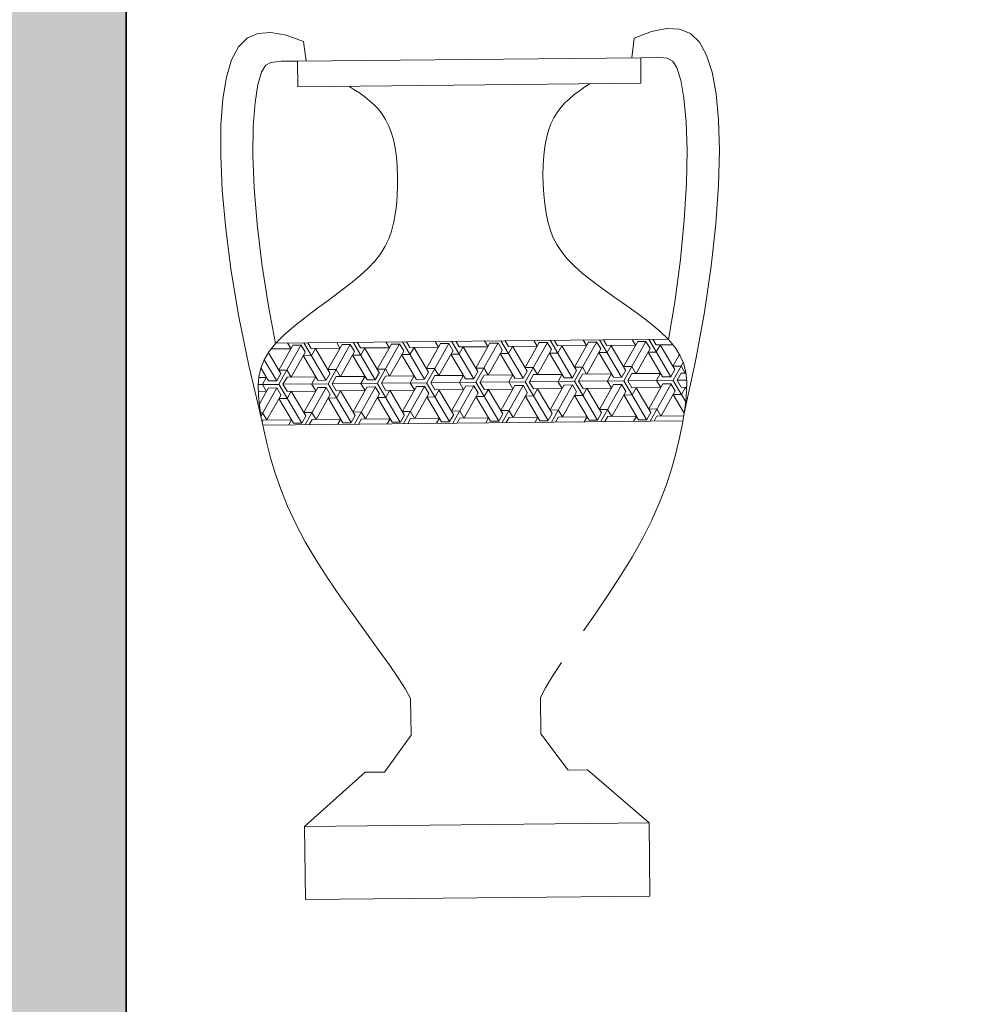
# Model space of a CAD drawing. Units: inches. Extents: x 638 to 1303, y 1 to 699.
# Tile 15 of 21: x 924.49 to 944.42, y 576.64 to 597.47. Entities that reach past the tile are written whole.
import ezdxf

# ---------------------------------------------------------------- set-up
doc = ezdxf.new("R2010")
doc.units = ezdxf.units.IN
doc.header["$MEASUREMENT"] = 0
doc.layers.add('A-FURN-ACCS', color=8, linetype='Continuous', lineweight=13)
doc.layers.add('A-WALL', color=7, linetype='Continuous', lineweight=35)
doc.layers.add('A-WALL-PATT', color=143, linetype='Continuous', lineweight=13, true_color=0x7aafdf)

msp = doc.modelspace()

# ---------------------------------------------------------------- hatches: boundary and pattern name
at = {"layer": 'A-WALL-PATT'}
h = msp.add_hatch(color=256, dxfattribs=at)
h.dxf.hatch_style = 1
h.paths.add_polyline_path([(973.34524, 629.81895), (793.35541, 629.81895), (793.35541, 620.81895), (850.23798, 620.81895), (922.23798, 620.81895), (922.23798, 524.81895), (908.94335, 524.81895), (908.94335, 520.31895), (926.73798, 520.31895), (926.73798, 544.31895), (979.3571, 544.31895), (979.3571, 548.81895), (926.73798, 548.81895), (926.73798, 620.81895), (973.34524, 620.81895)])
h.paths.add_polyline_path([(758.35541, 629.81895), (697.23798, 629.81895), (697.23798, 586.77451), (706.23798, 586.77451), (706.23798, 620.81895), (758.35541, 620.81895)])
h.paths.add_polyline_path([(1075.85281, 629.81895), (1003.34524, 629.81895), (1003.34524, 620.81895), (1046.73798, 620.81895), (1046.73798, 560.81895), (1046.73798, 548.81895), (1026.3571, 548.81895), (1026.3571, 544.31895), (1046.73798, 544.31895), (1046.73798, 486.87457), (1051.23798, 486.87457), (1051.23798, 556.31895), (1162.89753, 556.31895), (1162.89753, 560.81895), (1051.23798, 560.81895), (1051.23798, 620.81895), (1075.85281, 620.81895)])
h.paths.add_polyline_path([(1228.23798, 629.81895), (1105.85281, 629.81895), (1105.85281, 620.81895), (1219.23798, 620.81895), (1219.23798, 560.81895), (1197.89753, 560.81895), (1197.89753, 556.31895), (1219.23798, 556.31895), (1219.23798, 498.80084), (1228.23798, 498.80084)])
h.paths.add_polyline_path([(1051.23798, 439.87457), (1046.73798, 439.87457), (1046.73798, 407.81895), (1219.23798, 407.81895), (1219.23798, 381.66175), (1228.23798, 381.66175), (1228.23798, 451.80084), (1219.23798, 451.80084), (1219.23798, 412.31895), (1051.23798, 412.31895)])
h.paths.add_polyline_path([(1228.23798, 346.66175), (1219.23798, 346.66175), (1219.23798, 335.81895), (1046.73798, 335.81895), (1046.73798, 273.56895), (1051.23798, 273.56895), (1051.23798, 331.31895), (1219.23798, 331.31895), (1219.23798, 308.99654), (1228.23798, 308.99654)])
h.paths.add_polyline_path([(1228.23798, 261.99654), (1219.23798, 261.99654), (1219.23798, 211.31895), (1051.23798, 211.31895), (1051.23798, 226.56895), (1046.73798, 226.56895), (1046.73798, 211.31895), (983.84714, 211.31895), (983.84714, 206.81895), (1219.23798, 206.81895), (1219.23798, 166.83987), (1228.23798, 166.83987)])
h.paths.add_polyline_path([(1228.23798, 119.83987), (1219.23798, 119.83987), (1219.23798, 50.81895), (1197.89277, 50.81895), (1197.89277, 41.81895), (1228.23798, 41.81895)])
h.paths.add_polyline_path([(1162.89277, 50.81895), (1069.02949, 50.81895), (1069.02949, 41.81895), (1162.89277, 41.81895)])
h.paths.add_polyline_path([(1010.02949, 50.81895), (941.89631, 50.81895), (917.77455, 50.81895), (917.77455, 41.81895), (941.89631, 41.81895), (1010.02949, 41.81895)])
h.paths.add_polyline_path([(882.77455, 50.81895), (854.73798, 50.81895), (854.73798, 145.50379), (850.23798, 145.50379), (850.23798, 50.81895), (793.49755, 50.81895), (793.49755, 41.81895), (882.77455, 41.81895)])
h.paths.add_polyline_path([(746.49755, 50.81895), (706.23798, 50.81895), (706.23798, 96.57416), (697.23798, 96.57416), (697.23798, 41.81895), (746.49755, 41.81895)])
h.paths.add_polyline_path([(706.23798, 206.81895), (714.01165, 206.81895), (714.01165, 211.31895), (706.23798, 211.31895), (706.23798, 251.21966), (697.23798, 251.21966), (697.23798, 143.57416), (706.23798, 143.57416)])
h.paths.add_polyline_path([(923.84714, 211.31895), (854.73798, 211.31895), (854.73798, 397.8313), (850.23798, 397.8313), (850.23798, 388.31895), (747.9539, 388.31895), (747.9539, 383.81895), (850.23798, 383.81895), (850.23798, 311.81895), (706.23798, 311.81895), (706.23798, 342.78787), (697.23798, 342.78787), (697.23798, 281.21966), (706.23798, 281.21966), (706.23798, 307.31895), (850.23798, 307.31895), (850.23798, 211.31895), (749.01165, 211.31895), (749.01165, 206.81895), (850.23798, 206.81895), (850.23798, 192.50379), (854.73798, 192.50379), (854.73798, 206.81895), (923.84714, 206.81895)])
h.paths.add_polyline_path([(706.23798, 434.70471), (697.23798, 434.70471), (697.23798, 372.78787), (706.23798, 372.78787), (706.23798, 383.81895), (712.9539, 383.81895), (712.9539, 388.31895), (706.23798, 388.31895)])
h.paths.add_polyline_path([(706.23798, 520.31895), (850.23798, 520.31895), (850.23798, 444.8313), (854.73798, 444.8313), (854.73798, 520.31895), (861.94335, 520.31895), (861.94335, 524.81895), (706.23798, 524.81895), (706.23798, 551.77451), (697.23798, 551.77451), (697.23798, 481.70471), (706.23798, 481.70471)])

# ---------------------------------------------------------------- linework, layer by layer
at = {"layer": 'A-FURN-ACCS'}
for p, q in [((929.29851, 597.0812, 30.93634), (929.52655, 597.18264, 30.93634)), ((929.52655, 597.18264, 30.93634), (929.79966, 597.20234, 30.93634)), ((929.79966, 597.20234, 30.93634), (930.12044, 597.14336, 30.93634)), ((937.85335, 597.22234, 30.93634), (937.48516, 597.08018, 30.93634)), ((938.17285, 597.28786, 30.93634), (937.85335, 597.22234, 30.93634)), ((938.44632, 597.27375, 30.93634), (938.17285, 597.28786, 30.93634)), ((938.67638, 597.17698, 30.93634), (938.44632, 597.27375, 30.93634)), ((938.86569, 596.99458, 30.93634), (938.67638, 597.17698, 30.93634)), ((929.11296, 596.89496, 30.93634), (929.29851, 597.0812, 30.93634)), ((930.12044, 597.14336, 30.93634), (930.49145, 597.00875, 30.93634)), ((930.49145, 597.00875, 30.93634), (930.54731, 596.59361, 30.93634)), ((937.48516, 597.08018, 30.93634), (937.43779, 596.66399, 30.93634)), ((939.01689, 596.72351, 30.93634), (938.86569, 596.99458, 30.93634)), ((928.96733, 596.62087, 30.93634), (929.11296, 596.89496, 30.93634)), ((928.85903, 596.25587, 30.93634), (928.96733, 596.62087, 30.93634)), ((929.69512, 596.50919, 30.93634), (929.80088, 596.56912, 30.93634)), ((929.80088, 596.56912, 30.93634), (930.01698, 596.59481, 30.93634)), ((930.01698, 596.59481, 30.93634), (930.36281, 596.59173, 30.93634)), ((930.36281, 596.59173, 30.93634), (933.99255, 596.6288, 30.93634)), ((930.36831, 596.05264, 30.93634), (930.36281, 596.59173, 30.93634)), ((937.6223, 596.66587, 30.93634), (933.99255, 596.6288, 30.93634)), ((937.968, 596.67602, 30.93634), (937.6223, 596.66587, 30.93634)), ((937.62781, 596.12679, 30.93634), (937.6223, 596.66587, 30.93634)), ((938.18458, 596.65474, 30.93634), (937.968, 596.67602, 30.93634)), ((938.29153, 596.59699, 30.93634), (938.18458, 596.65474, 30.93634)), ((938.29373, 596.59607, 30.93634), (938.29153, 596.59699, 30.93634)), ((938.31801, 596.57267, 30.93634), (938.29373, 596.59607, 30.93634)), ((938.38627, 596.45029, 30.93634), (938.31801, 596.57267, 30.93634)), ((939.13263, 596.3608, 30.93634), (939.01689, 596.72351, 30.93634)), ((929.52722, 596.10387, 30.93634), (929.6034, 596.36059, 30.93634)), ((929.6034, 596.36059, 30.93634), (929.66915, 596.48434, 30.93634)), ((929.66915, 596.48434, 30.93634), (929.69295, 596.50823, 30.93634)), ((929.69295, 596.50823, 30.93634), (929.69512, 596.50919, 30.93634)), ((938.46767, 596.19518, 30.93634), (938.38627, 596.45029, 30.93634)), ((939.21554, 595.90342, 30.93634), (939.13263, 596.3608, 30.93634)), ((928.78547, 595.79689, 30.93634), (928.85903, 596.25587, 30.93634)), ((938.53745, 595.81025, 30.93634), (938.46767, 596.19518, 30.93634)), ((929.46532, 595.71759, 30.93634), (929.52722, 596.10387, 30.93634)), ((937.62781, 596.12679, 30.93634), (930.36831, 596.05264, 30.93634)), ((931.55847, 595.99769, 30.93634), (931.44982, 596.06369, 30.93634)), ((931.67465, 595.92083, 30.93634), (931.55847, 595.99769, 30.93634)), ((936.21523, 595.88586, 30.93634), (936.32443, 595.96832, 30.93634)), ((936.32443, 595.96832, 30.93634), (936.43902, 596.04754, 30.93634)), ((936.43902, 596.04754, 30.93634), (936.5463, 596.11574, 30.93634)), ((928.74499, 595.24222, 30.93634), (928.78547, 595.79689, 30.93634)), ((929.42832, 595.21387, 30.93634), (929.46532, 595.71759, 30.93634)), ((931.78552, 595.84061, 30.93634), (931.67465, 595.92083, 30.93634)), ((931.88949, 595.75738, 30.93634), (931.78552, 595.84061, 30.93634)), ((931.98601, 595.66959, 30.93634), (931.88949, 595.75738, 30.93634)), ((936.01827, 595.71078, 30.93634), (936.11298, 595.80052, 30.93634)), ((936.11298, 595.80052, 30.93634), (936.21523, 595.88586, 30.93634)), ((938.58474, 595.30739, 30.93634), (938.53745, 595.81025, 30.93634)), ((939.26735, 595.34969, 30.93634), (939.21554, 595.90342, 30.93634)), ((932.07478, 595.57522, 30.93634), (931.98601, 595.66959, 30.93634)), ((932.1555, 595.47224, 30.93634), (932.07478, 595.57522, 30.93634)), ((935.78282, 595.39495, 30.93634), (935.85285, 595.51, 30.93634)), ((935.85285, 595.51, 30.93634), (935.93144, 595.61461, 30.93634)), ((935.93144, 595.61461, 30.93634), (936.01827, 595.71078, 30.93634)), ((932.22786, 595.35864, 30.93634), (932.1555, 595.47224, 30.93634)), ((932.29156, 595.23239, 30.93634), (932.22786, 595.35864, 30.93634)), ((935.72171, 595.26743, 30.93634), (935.78282, 595.39495, 30.93634)), ((938.60375, 594.70267, 30.93634), (938.58474, 595.30739, 30.93634)), ((939.28607, 594.70319, 30.93634), (939.26735, 595.34969, 30.93634)), ((928.73948, 594.59548, 30.93634), (928.74499, 595.24222, 30.93634)), ((929.42167, 594.60889, 30.93634), (929.42832, 595.21387, 30.93634)), ((932.3463, 595.09149, 30.93634), (932.29156, 595.23239, 30.93634)), ((932.39177, 594.9339, 30.93634), (932.3463, 595.09149, 30.93634)), ((935.62762, 594.96695, 30.93634), (935.66987, 595.12543, 30.93634)), ((935.66987, 595.12543, 30.93634), (935.72171, 595.26743, 30.93634)), ((932.42776, 594.75862, 30.93634), (932.39177, 594.9339, 30.93634)), ((935.59522, 594.79097, 30.93634), (935.62762, 594.96695, 30.93634)), ((932.4544, 594.56868, 30.93634), (932.42776, 594.75862, 30.93634)), ((935.57246, 594.60053, 30.93634), (935.59522, 594.79097, 30.93634)), ((938.5911, 594.00917, 30.93634), (938.60375, 594.70267, 30.93634)), ((939.2688, 593.96883, 30.93634), (939.28607, 594.70319, 30.93634)), ((928.77174, 593.86162, 30.93634), (928.73948, 594.59548, 30.93634)), ((929.44847, 593.91579, 30.93634), (929.42167, 594.60889, 30.93634)), ((932.47192, 594.36811, 30.93634), (932.4544, 594.56868, 30.93634)), ((935.55904, 594.39964, 30.93634), (935.57246, 594.60053, 30.93634)), ((932.48054, 594.16097, 30.93634), (932.47192, 594.36811, 30.93634)), ((935.55466, 594.19236, 30.93634), (935.55904, 594.39964, 30.93634)), ((932.48047, 593.95127, 30.93634), (932.48054, 594.16097, 30.93634)), ((935.55902, 593.98272, 30.93634), (935.55466, 594.19236, 30.93634)), ((928.84459, 593.0456, 30.93634), (928.77174, 593.86162, 30.93634)), ((929.51085, 593.14522, 30.93634), (929.44847, 593.91579, 30.93634)), ((932.47193, 593.74308, 30.93634), (932.48047, 593.95127, 30.93634)), ((935.5718, 593.77474, 30.93634), (935.55902, 593.98272, 30.93634)), ((938.54447, 593.23749, 30.93634), (938.5911, 594.00917, 30.93634)), ((939.21263, 593.1515, 30.93634), (939.2688, 593.96883, 30.93634)), ((932.45516, 593.54042, 30.93634), (932.47193, 593.74308, 30.93634)), ((935.59271, 593.57246, 30.93634), (935.5718, 593.77474, 30.93634)), ((932.43036, 593.34733, 30.93634), (932.45516, 593.54042, 30.93634)), ((935.62144, 593.37993, 30.93634), (935.59271, 593.57246, 30.93634)), ((932.39722, 593.16674, 30.93634), (932.43036, 593.34733, 30.93634)), ((935.65827, 593.20005, 30.93634), (935.62144, 593.37993, 30.93634)), ((938.46194, 592.39714, 30.93634), (938.54447, 593.23749, 30.93634)), ((928.96082, 592.15238, 30.93634), (928.84459, 593.0456, 30.93634)), ((929.61053, 592.30674, 30.93634), (929.51085, 593.14522, 30.93634)), ((932.35318, 592.99706, 30.93634), (932.39722, 593.16674, 30.93634)), ((935.70577, 593.0313, 30.93634), (935.65827, 593.20005, 30.93634)), ((935.76708, 592.87105, 30.93634), (935.70577, 593.0313, 30.93634)), ((939.11467, 592.25609, 30.93634), (939.21263, 593.1515, 30.93634)), ((932.22003, 592.67962, 30.93634), (932.29515, 592.83558, 30.93634)), ((932.29515, 592.83558, 30.93634), (932.35318, 592.99706, 30.93634)), ((935.84537, 592.71665, 30.93634), (935.76708, 592.87105, 30.93634)), ((932.12473, 592.52646, 30.93634), (932.22003, 592.67962, 30.93634)), ((935.94378, 592.56547, 30.93634), (935.84537, 592.71665, 30.93634)), ((932.00616, 592.3734, 30.93634), (932.12473, 592.52646, 30.93634)), ((936.06546, 592.41486, 30.93634), (935.94378, 592.56547, 30.93634)), ((936.21355, 592.2622, 30.93634), (936.06546, 592.41486, 30.93634)), ((938.34177, 591.49707, 30.93634), (938.46194, 592.39714, 30.93634)), ((929.74906, 591.40931, 30.93634), (929.61053, 592.30674, 30.93634)), ((931.68679, 592.05679, 30.93634), (931.86121, 592.21775, 30.93634)), ((931.86121, 592.21775, 30.93634), (932.00616, 592.3734, 30.93634)), ((936.39122, 592.10484, 30.93634), (936.21355, 592.2622, 30.93634)), ((938.972, 591.28751, 30.93634), (939.11467, 592.25609, 30.93634)), ((929.12324, 591.18692, 30.93634), (928.96082, 592.15238, 30.93634)), ((931.48184, 591.88855, 30.93634), (931.68679, 592.05679, 30.93634)), ((936.59956, 591.94082, 30.93634), (936.39122, 592.10484, 30.93634)), ((931.25343, 591.71392, 30.93634), (931.48184, 591.88855, 30.93634)), ((936.83149, 591.77089, 30.93634), (936.59956, 591.94082, 30.93634)), ((937.07788, 591.59648, 30.93634), (936.83149, 591.77089, 30.93634)), ((931.01066, 591.53451, 30.93634), (931.25343, 591.71392, 30.93634)), ((937.32958, 591.41902, 30.93634), (937.07788, 591.59648, 30.93634)), ((929.89803, 590.61989, 30.93634), (929.74906, 591.40931, 30.93634)), ((930.51846, 591.16783, 30.93634), (930.76264, 591.35194, 30.93634)), ((930.76264, 591.35194, 30.93634), (931.01066, 591.53451, 30.93634)), ((937.57747, 591.23993, 30.93634), (937.32958, 591.41902, 30.93634)), ((938.20896, 590.70478, 30.93634), (938.34177, 591.49707, 30.93634)), ((929.33466, 590.15416, 30.93634), (929.12324, 591.18692, 30.93634)), ((930.28722, 590.98379, 30.93634), (930.51846, 591.16783, 30.93634)), ((937.81241, 591.06065, 30.93634), (937.57747, 591.23993, 30.93634)), ((938.78172, 590.25065, 30.93634), (938.972, 591.28751, 30.93634)), ((930.07804, 590.80143, 30.93634), (930.28722, 590.98379, 30.93634)), ((938.02528, 590.8826, 30.93634), (937.81241, 591.06065, 30.93634)), ((929.90001, 590.62237, 30.93634), (930.07804, 590.80143, 30.93634)), ((929.90745, 590.62986, 30.93634), (938.19933, 590.71455, 30.93634)), ((938.20692, 590.70722, 30.93634), (938.02528, 590.8826, 30.93634)), ((929.76011, 590.44736, 30.93634), (929.90001, 590.62237, 30.93634)), ((929.80815, 590.50746, 30.93634), (930.22084, 590.51168, 30.93634)), ((930.26494, 590.58895, 30.93634), (929.96637, 590.05939, 30.93634)), ((929.96944, 589.75857, 30.93634), (930.43863, 590.59072, 30.93634)), ((930.15006, 590.63234, 30.93634), (930.22016, 590.51374, 30.93634)), ((930.43718, 590.5891, 30.93634), (930.26349, 590.58733, 30.93634)), ((930.43649, 590.59117, 30.93634), (930.52487, 590.44164, 30.93634)), ((930.49743, 590.63588, 30.93634), (930.96523, 589.84442, 30.93634)), ((930.58427, 590.63677, 30.93634), (930.65437, 590.51818, 30.93634)), ((930.65505, 590.51611, 30.93634), (931.26294, 590.52232, 30.93634)), ((930.65804, 590.36732, 30.93634), (930.74334, 590.51862, 30.93634)), ((931.05053, 589.99572, 30.93634), (930.74121, 590.51907, 30.93634)), ((931.30705, 590.59959, 30.93634), (931.00848, 590.07004, 30.93634)), ((931.01155, 589.76921, 30.93634), (931.48073, 590.60137, 30.93634)), ((931.19217, 590.64298, 30.93634), (931.26226, 590.52439, 30.93634)), ((931.47928, 590.59974, 30.93634), (931.3056, 590.59797, 30.93634)), ((931.4786, 590.60181, 30.93634), (931.56698, 590.45229, 30.93634)), ((931.53954, 590.64653, 30.93634), (932.00733, 589.85506, 30.93634)), ((931.62638, 590.64741, 30.93634), (931.69647, 590.52882, 30.93634)), ((931.69715, 590.52675, 30.93634), (932.30505, 590.53296, 30.93634)), ((931.70014, 590.37796, 30.93634), (931.78545, 590.52926, 30.93634)), ((932.09264, 590.00636, 30.93634), (931.78331, 590.52971, 30.93634)), ((932.34915, 590.61024, 30.93634), (932.05058, 590.08068, 30.93634)), ((932.05366, 589.77985, 30.93634), (932.52284, 590.61201, 30.93634)), ((932.23428, 590.65362, 30.93634), (932.30437, 590.53503, 30.93634)), ((932.52138, 590.61039, 30.93634), (932.3477, 590.60861, 30.93634)), ((932.52071, 590.61246, 30.93634), (932.60908, 590.46293, 30.93634)), ((932.58164, 590.65717, 30.93634), (933.04944, 589.86571, 30.93634)), ((932.66849, 590.65806, 30.93634), (932.73858, 590.53947, 30.93634)), ((932.73926, 590.5374, 30.93634), (933.34715, 590.54361, 30.93634)), ((932.74225, 590.38861, 30.93634), (932.82755, 590.53991, 30.93634)), ((933.13474, 590.01701, 30.93634), (932.82542, 590.54036, 30.93634)), ((933.39126, 590.62088, 30.93634), (933.09269, 590.09132, 30.93634)), ((933.09576, 589.79049, 30.93634), (933.56494, 590.62265, 30.93634)), ((933.27638, 590.66427, 30.93634), (933.34647, 590.54568, 30.93634)), ((933.56349, 590.62103, 30.93634), (933.3898, 590.61926, 30.93634)), ((933.56281, 590.6231, 30.93634), (933.65119, 590.47358, 30.93634)), ((933.62375, 590.66781, 30.93634), (934.09154, 589.87635, 30.93634)), ((933.71059, 590.6687, 30.93634), (933.78068, 590.55011, 30.93634)), ((933.78136, 590.54804, 30.93634), (934.38926, 590.55425, 30.93634)), ((933.78435, 590.39925, 30.93634), (933.86966, 590.55055, 30.93634)), ((934.17685, 590.02765, 30.93634), (933.86753, 590.551, 30.93634)), ((934.43337, 590.63152, 30.93634), (934.1348, 590.10197, 30.93634)), ((934.13787, 589.80114, 30.93634), (934.60705, 590.6333, 30.93634)), ((934.31849, 590.67491, 30.93634), (934.38858, 590.55632, 30.93634)), ((934.60559, 590.63168, 30.93634), (934.43191, 590.6299, 30.93634)), ((934.60492, 590.63375, 30.93634), (934.6933, 590.48422, 30.93634)), ((934.66586, 590.67846, 30.93634), (935.13365, 589.887, 30.93634)), ((934.7527, 590.67935, 30.93634), (934.82279, 590.56076, 30.93634)), ((934.82347, 590.55868, 30.93634), (935.43136, 590.56489, 30.93634)), ((934.82646, 590.40989, 30.93634), (934.91177, 590.56119, 30.93634)), ((935.21896, 590.0383, 30.93634), (934.90963, 590.56164, 30.93634)), ((935.47547, 590.64217, 30.93634), (935.1769, 590.11261, 30.93634)), ((935.17997, 589.81178, 30.93634), (935.64916, 590.64394, 30.93634)), ((935.3606, 590.68555, 30.93634), (935.43069, 590.56697, 30.93634)), ((935.6477, 590.64232, 30.93634), (935.47401, 590.64054, 30.93634)), ((935.64702, 590.64439, 30.93634), (935.7354, 590.49486, 30.93634)), ((935.70796, 590.6891, 30.93634), (936.17576, 589.89764, 30.93634)), ((935.79481, 590.68999, 30.93634), (935.8649, 590.5714, 30.93634)), ((935.86557, 590.56933, 30.93634), (936.47347, 590.57554, 30.93634)), ((935.86857, 590.42053, 30.93634), (935.95387, 590.57184, 30.93634)), ((936.26106, 590.04894, 30.93634), (935.95174, 590.57229, 30.93634)), ((936.51758, 590.65281, 30.93634), (936.21901, 590.12325, 30.93634)), ((936.22208, 589.82242, 30.93634), (936.69126, 590.65458, 30.93634)), ((936.4027, 590.6962, 30.93634), (936.47279, 590.57761, 30.93634)), ((936.6898, 590.65296, 30.93634), (936.51612, 590.65119, 30.93634)), ((936.68913, 590.65504, 30.93634), (936.77751, 590.50551, 30.93634)), ((936.75007, 590.69975, 30.93634), (937.21786, 589.90828, 30.93634)), ((936.83691, 590.70063, 30.93634), (936.907, 590.58205, 30.93634)), ((936.90768, 590.57997, 30.93634), (937.51557, 590.58618, 30.93634)), ((936.91067, 590.43118, 30.93634), (936.99598, 590.58248, 30.93634)), ((937.30317, 590.05959, 30.93634), (936.99384, 590.58293, 30.93634)), ((937.55968, 590.66345, 30.93634), (937.26111, 590.1339, 30.93634)), ((937.26419, 589.83307, 30.93634), (937.73337, 590.66523, 30.93634)), ((937.44481, 590.70684, 30.93634), (937.5149, 590.58826, 30.93634)), ((937.82175, 590.5157, 30.93634), (937.52318, 589.98614, 30.93634)), ((937.73191, 590.66361, 30.93634), (937.55822, 590.66183, 30.93634)), ((937.73123, 590.66568, 30.93634), (937.81961, 590.51615, 30.93634)), ((937.79218, 590.71039, 30.93634), (938.25997, 589.91893, 30.93634)), ((937.87902, 590.71128, 30.93634), (937.94911, 590.59269, 30.93634)), ((937.94978, 590.59062, 30.93634), (938.30111, 590.5942, 30.93634)), ((937.95278, 590.44182, 30.93634), (938.03808, 590.59312, 30.93634)), ((938.34527, 590.07023, 30.93634), (938.03595, 590.59358, 30.93634)), ((938.35037, 590.5351, 30.93634), (938.20692, 590.70722, 30.93634)), ((938.45724, 590.36357, 30.93634), (938.35037, 590.5351, 30.93634)), ((929.65677, 590.27368, 30.93634), (929.76011, 590.44736, 30.93634)), ((930.00843, 589.98507, 30.93634), (929.74761, 590.42635, 30.93634)), ((930.527, 590.4412, 30.93634), (930.22843, 589.91164, 30.93634)), ((930.79154, 589.84264, 30.93634), (930.48222, 590.36599, 30.93634)), ((930.65658, 590.3657, 30.93634), (930.4829, 590.36392, 30.93634)), ((931.56911, 590.45184, 30.93634), (931.27054, 589.92228, 30.93634)), ((931.83365, 589.85329, 30.93634), (931.52432, 590.37664, 30.93634)), ((931.69869, 590.37634, 30.93634), (931.52501, 590.37457, 30.93634)), ((932.61122, 590.46248, 30.93634), (932.31265, 589.93293, 30.93634)), ((932.87575, 589.86393, 30.93634), (932.56643, 590.38728, 30.93634)), ((932.74079, 590.38698, 30.93634), (932.56711, 590.38521, 30.93634)), ((933.65332, 590.47313, 30.93634), (933.35475, 589.94357, 30.93634)), ((933.91786, 589.87458, 30.93634), (933.60854, 590.39792, 30.93634)), ((933.7829, 590.39763, 30.93634), (933.60921, 590.39585, 30.93634)), ((934.69543, 590.48377, 30.93634), (934.39686, 589.95421, 30.93634)), ((934.95997, 589.88522, 30.93634), (934.65064, 590.40857, 30.93634)), ((934.825, 590.40827, 30.93634), (934.65132, 590.4065, 30.93634)), ((935.73753, 590.49441, 30.93634), (935.43896, 589.96486, 30.93634)), ((936.00207, 589.89587, 30.93634), (935.69275, 590.41921, 30.93634)), ((935.86711, 590.41891, 30.93634), (935.69342, 590.41714, 30.93634)), ((936.77964, 590.50505, 30.93634), (936.48107, 589.9755, 30.93634)), ((937.04418, 589.90651, 30.93634), (936.73485, 590.42986, 30.93634)), ((936.90921, 590.42956, 30.93634), (936.73553, 590.42778, 30.93634)), ((938.08628, 589.91715, 30.93634), (937.77696, 590.4405, 30.93634)), ((937.95132, 590.4402, 30.93634), (937.77763, 590.43843, 30.93634)), ((938.44121, 590.38929, 30.93634), (938.30322, 590.14454, 30.93634)), ((938.53129, 590.18912, 30.93634), (938.45724, 590.36357, 30.93634)), ((929.59788, 589.05908, 30.93634), (929.33466, 590.15416, 30.93634)), ((929.54502, 589.916, 30.93634), (929.5863, 590.09776, 30.93634)), ((929.5863, 590.09776, 30.93634), (929.65677, 590.27368, 30.93634)), ((929.74944, 589.832, 30.93634), (929.58875, 590.10387, 30.93634)), ((929.65995, 590.27903, 30.93634), (929.92312, 589.83377, 30.93634)), ((933.26492, 590.09147, 30.93634), (933.09123, 590.0897, 30.93634)), ((933.26424, 590.09355, 30.93634), (933.35262, 589.94402, 30.93634)), ((934.30702, 590.10212, 30.93634), (934.13334, 590.10034, 30.93634)), ((934.30635, 590.10419, 30.93634), (934.39472, 589.95466, 30.93634)), ((935.34913, 590.11276, 30.93634), (935.17544, 590.11099, 30.93634)), ((935.34845, 590.11484, 30.93634), (935.43683, 589.96531, 30.93634)), ((936.39123, 590.1234, 30.93634), (936.21755, 590.12163, 30.93634)), ((936.39056, 590.12548, 30.93634), (936.47894, 589.97595, 30.93634)), ((937.43334, 590.13405, 30.93634), (937.25965, 590.13227, 30.93634)), ((937.43266, 590.13612, 30.93634), (937.52104, 589.9866, 30.93634)), ((938.47544, 590.14469, 30.93634), (938.30176, 590.14292, 30.93634)), ((938.30629, 589.84371, 30.93634), (938.51829, 590.21972, 30.93634)), ((938.47477, 590.14677, 30.93634), (938.56315, 589.99724, 30.93634)), ((938.57627, 590.00824, 30.93634), (938.53129, 590.18912, 30.93634)), ((938.54093, 589.15042, 30.93634), (938.78172, 590.25065, 30.93634)), ((929.52922, 589.72483, 30.93634), (929.54502, 589.916, 30.93634)), ((929.54395, 589.90304, 30.93634), (929.70593, 589.90469, 30.93634)), ((929.62208, 589.75502, 30.93634), (929.70738, 589.90632, 30.93634)), ((929.92526, 589.83333, 30.93634), (930.01056, 589.98463, 30.93634)), ((930.13861, 590.05954, 30.93634), (929.96492, 590.05777, 30.93634)), ((930.05629, 589.75945, 30.93634), (930.14159, 589.91075, 30.93634)), ((930.13792, 590.06161, 30.93634), (930.2263, 589.91208, 30.93634)), ((930.14014, 589.90913, 30.93634), (930.74804, 589.91534, 30.93634)), ((930.66418, 589.76566, 30.93634), (930.74949, 589.91696, 30.93634)), ((930.96736, 589.84397, 30.93634), (931.05267, 589.99527, 30.93634)), ((931.18071, 590.07019, 30.93634), (931.00703, 590.06841, 30.93634)), ((931.09839, 589.77009, 30.93634), (931.1837, 589.9214, 30.93634)), ((931.18003, 590.07226, 30.93634), (931.26841, 589.92273, 30.93634)), ((931.18225, 589.91977, 30.93634), (931.79014, 589.92598, 30.93634)), ((931.70629, 589.7763, 30.93634), (931.79159, 589.9276, 30.93634)), ((932.00947, 589.85461, 30.93634), (932.09477, 590.00592, 30.93634)), ((932.22281, 590.08083, 30.93634), (932.04913, 590.07906, 30.93634)), ((932.1405, 589.78074, 30.93634), (932.2258, 589.93204, 30.93634)), ((932.22213, 590.0829, 30.93634), (932.31051, 589.93337, 30.93634)), ((932.22435, 589.93041, 30.93634), (932.83224, 589.93662, 30.93634)), ((932.74839, 589.78695, 30.93634), (932.8337, 589.93825, 30.93634)), ((933.05157, 589.86526, 30.93634), (933.13688, 590.01656, 30.93634)), ((933.1826, 589.79138, 30.93634), (933.26791, 589.94268, 30.93634)), ((933.26645, 589.94106, 30.93634), (933.87435, 589.94727, 30.93634)), ((933.7905, 589.79759, 30.93634), (933.87581, 589.94889, 30.93634)), ((934.09368, 589.8759, 30.93634), (934.17898, 590.0272, 30.93634)), ((934.22471, 589.80202, 30.93634), (934.31002, 589.95333, 30.93634)), ((934.30856, 589.9517, 30.93634), (934.91645, 589.95791, 30.93634)), ((934.83261, 589.80823, 30.93634), (934.91791, 589.95953, 30.93634)), ((935.13433, 589.88492, 30.93634), (934.96064, 589.88315, 30.93634)), ((935.13579, 589.88654, 30.93634), (935.22109, 590.03785, 30.93634)), ((935.26682, 589.81267, 30.93634), (935.35212, 589.96397, 30.93634)), ((935.35066, 589.96235, 30.93634), (935.95856, 589.96855, 30.93634)), ((935.87471, 589.81887, 30.93634), (935.96002, 589.97018, 30.93634)), ((936.17643, 589.89556, 30.93634), (936.00275, 589.89379, 30.93634)), ((936.17789, 589.89719, 30.93634), (936.2632, 590.04849, 30.93634)), ((936.30892, 589.82331, 30.93634), (936.39423, 589.97461, 30.93634)), ((936.39277, 589.97299, 30.93634), (937.00066, 589.9792, 30.93634)), ((936.91682, 589.82952, 30.93634), (937.00212, 589.98082, 30.93634)), ((937.21854, 589.90621, 30.93634), (937.04485, 589.90443, 30.93634)), ((937.22, 589.90783, 30.93634), (937.3053, 590.05913, 30.93634)), ((937.35103, 589.83395, 30.93634), (937.43633, 589.98525, 30.93634)), ((937.43487, 589.98363, 30.93634), (938.04277, 589.98984, 30.93634)), ((937.95892, 589.84016, 30.93634), (938.04423, 589.99146, 30.93634)), ((938.26064, 589.91685, 30.93634), (938.08696, 589.91508, 30.93634)), ((938.2621, 589.91847, 30.93634), (938.34741, 590.06977, 30.93634)), ((938.39313, 589.8446, 30.93634), (938.47844, 589.9959, 30.93634)), ((938.47698, 589.99428, 30.93634), (938.57761, 589.99531, 30.93634)), ((938.57489, 590.01382, 30.93634), (938.56528, 589.99678, 30.93634)), ((938.59597, 589.81744, 30.93634), (938.57627, 590.00824, 30.93634)), ((929.53523, 589.52068, 30.93634), (929.52922, 589.72483, 30.93634)), ((929.96799, 589.75694, 30.93634), (929.53151, 589.75248, 30.93634)), ((929.75311, 589.68114, 30.93634), (929.55591, 589.33138, 30.93634)), ((929.59283, 589.09059, 30.93634), (929.92679, 589.68291, 30.93634)), ((929.61994, 589.75546, 30.93634), (929.70832, 589.60593, 30.93634)), ((929.9238, 589.8317, 30.93634), (929.75012, 589.82993, 30.93634)), ((929.92534, 589.68129, 30.93634), (929.75166, 589.67951, 30.93634)), ((929.92466, 589.68336, 30.93634), (930.01304, 589.53383, 30.93634)), ((929.96731, 589.75901, 30.93634), (930.45339, 588.93661, 30.93634)), ((930.05415, 589.7599, 30.93634), (930.14253, 589.61037, 30.93634)), ((931.0101, 589.76758, 30.93634), (930.05484, 589.75783, 30.93634)), ((930.79521, 589.69178, 30.93634), (930.49664, 589.16223, 30.93634)), ((930.52464, 588.90561, 30.93634), (930.9689, 589.69356, 30.93634)), ((930.66205, 589.76611, 30.93634), (930.75043, 589.61658, 30.93634)), ((930.96591, 589.84235, 30.93634), (930.79222, 589.84057, 30.93634)), ((930.96745, 589.69193, 30.93634), (930.79376, 589.69016, 30.93634)), ((930.96676, 589.694, 30.93634), (931.05514, 589.54447, 30.93634)), ((931.00942, 589.76965, 30.93634), (931.4955, 588.94725, 30.93634)), ((931.09626, 589.77054, 30.93634), (931.18464, 589.62101, 30.93634)), ((932.0522, 589.77823, 30.93634), (931.09694, 589.76847, 30.93634)), ((931.83732, 589.70243, 30.93634), (931.53875, 589.17287, 30.93634)), ((931.56675, 588.91625, 30.93634), (932.011, 589.7042, 30.93634)), ((931.70415, 589.77675, 30.93634), (931.79253, 589.62722, 30.93634)), ((932.00801, 589.85299, 30.93634), (931.83433, 589.85122, 30.93634)), ((932.00955, 589.70258, 30.93634), (931.83587, 589.7008, 30.93634)), ((932.00887, 589.70465, 30.93634), (932.09725, 589.55512, 30.93634)), ((932.05152, 589.7803, 30.93634), (932.5376, 588.95789, 30.93634)), ((932.13836, 589.78118, 30.93634), (932.22674, 589.63166, 30.93634)), ((933.09431, 589.78887, 30.93634), (932.13904, 589.77911, 30.93634)), ((932.87943, 589.71307, 30.93634), (932.58086, 589.18351, 30.93634)), ((932.60885, 588.92689, 30.93634), (933.05311, 589.71484, 30.93634)), ((932.74626, 589.78739, 30.93634), (932.83464, 589.63787, 30.93634)), ((933.05012, 589.86363, 30.93634), (932.87643, 589.86186, 30.93634)), ((933.05165, 589.71322, 30.93634), (932.87797, 589.71145, 30.93634)), ((933.05098, 589.71529, 30.93634), (933.13935, 589.56576, 30.93634)), ((933.09363, 589.79094, 30.93634), (933.57971, 588.96854, 30.93634)), ((933.18047, 589.79183, 30.93634), (933.26885, 589.6423, 30.93634)), ((934.13641, 589.79951, 30.93634), (933.18115, 589.78976, 30.93634)), ((933.92153, 589.72371, 30.93634), (933.62296, 589.19416, 30.93634)), ((933.65096, 588.93754, 30.93634), (934.09522, 589.72549, 30.93634)), ((933.78837, 589.79804, 30.93634), (933.87674, 589.64851, 30.93634)), ((934.09222, 589.87428, 30.93634), (933.91854, 589.8725, 30.93634)), ((934.09376, 589.72386, 30.93634), (933.92007, 589.72209, 30.93634)), ((934.09308, 589.72594, 30.93634), (934.18146, 589.57641, 30.93634)), ((934.13573, 589.80159, 30.93634), (934.62181, 588.97918, 30.93634)), ((934.22258, 589.80247, 30.93634), (934.31095, 589.65295, 30.93634)), ((935.17852, 589.81016, 30.93634), (934.22325, 589.8004, 30.93634)), ((934.96364, 589.73436, 30.93634), (934.66507, 589.2048, 30.93634)), ((934.69307, 588.94818, 30.93634), (935.13732, 589.73613, 30.93634)), ((934.83047, 589.80868, 30.93634), (934.91885, 589.65916, 30.93634)), ((935.13586, 589.73451, 30.93634), (934.96218, 589.73273, 30.93634)), ((935.13519, 589.73658, 30.93634), (935.22357, 589.58705, 30.93634)), ((935.17784, 589.81223, 30.93634), (935.66392, 588.98983, 30.93634)), ((935.26468, 589.81312, 30.93634), (935.35306, 589.66359, 30.93634)), ((936.22062, 589.8208, 30.93634), (935.26536, 589.81104, 30.93634)), ((936.00574, 589.745, 30.93634), (935.70717, 589.21544, 30.93634)), ((935.73517, 588.95882, 30.93634), (936.17943, 589.74677, 30.93634)), ((935.87258, 589.81933, 30.93634), (935.96096, 589.6698, 30.93634)), ((936.17797, 589.74515, 30.93634), (936.00428, 589.74338, 30.93634)), ((936.17729, 589.74723, 30.93634), (936.26567, 589.5977, 30.93634)), ((936.21995, 589.82288, 30.93634), (936.70603, 589.00047, 30.93634)), ((936.30679, 589.82376, 30.93634), (936.39517, 589.67424, 30.93634)), ((937.26272, 589.83144, 30.93634), (936.30746, 589.82169, 30.93634)), ((936.39584, 589.67216, 30.93634), (937.00374, 589.67837, 30.93634)), ((936.39884, 589.52337, 30.93634), (936.48414, 589.67467, 30.93634)), ((936.79133, 589.15177, 30.93634), (936.48201, 589.67512, 30.93634)), ((937.04785, 589.75564, 30.93634), (936.74928, 589.22608, 30.93634)), ((936.77728, 588.96947, 30.93634), (937.22153, 589.75741, 30.93634)), ((936.91468, 589.82997, 30.93634), (937.00306, 589.68044, 30.93634)), ((937.22007, 589.75579, 30.93634), (937.04639, 589.75402, 30.93634)), ((937.2194, 589.75787, 30.93634), (937.30778, 589.60834, 30.93634)), ((937.26205, 589.83352, 30.93634), (937.74813, 589.01112, 30.93634)), ((937.34889, 589.83441, 30.93634), (937.43727, 589.68488, 30.93634)), ((938.30483, 589.84209, 30.93634), (937.34957, 589.83233, 30.93634)), ((937.43795, 589.6828, 30.93634), (938.04584, 589.68901, 30.93634)), ((937.44094, 589.53401, 30.93634), (937.52625, 589.68531, 30.93634)), ((937.83344, 589.16242, 30.93634), (937.52411, 589.68577, 30.93634)), ((938.08995, 589.76628, 30.93634), (937.79138, 589.23673, 30.93634)), ((937.81939, 588.98011, 30.93634), (938.26364, 589.76806, 30.93634)), ((937.95679, 589.84062, 30.93634), (938.04517, 589.69109, 30.93634)), ((938.26218, 589.76644, 30.93634), (938.08849, 589.76466, 30.93634)), ((938.2615, 589.76851, 30.93634), (938.34988, 589.61899, 30.93634)), ((938.30416, 589.84416, 30.93634), (938.57393, 589.38773, 30.93634)), ((938.391, 589.84505, 30.93634), (938.47938, 589.69552, 30.93634)), ((938.59312, 589.84503, 30.93634), (938.39167, 589.84298, 30.93634)), ((938.48005, 589.69345, 30.93634), (938.59487, 589.69462, 30.93634)), ((938.48305, 589.54465, 30.93634), (938.56835, 589.69595, 30.93634)), ((938.59445, 589.64864, 30.93634), (938.56622, 589.69641, 30.93634)), ((938.59413, 589.6132, 30.93634), (938.59597, 589.81744, 30.93634)), ((929.53284, 589.60206, 30.93634), (929.709, 589.60386, 30.93634)), ((929.55934, 589.29996, 30.93634), (929.53523, 589.52068, 30.93634)), ((930.01517, 589.53339, 30.93634), (929.7166, 589.00383, 30.93634)), ((930.14321, 589.6083, 30.93634), (930.75111, 589.61451, 30.93634)), ((930.1462, 589.45951, 30.93634), (930.23151, 589.61081, 30.93634)), ((930.5387, 589.08791, 30.93634), (930.22937, 589.61125, 30.93634)), ((931.05728, 589.54403, 30.93634), (930.75871, 589.01447, 30.93634)), ((931.32181, 588.94548, 30.93634), (931.01249, 589.46882, 30.93634)), ((931.18685, 589.46853, 30.93634), (931.01317, 589.46675, 30.93634)), ((931.18532, 589.61894, 30.93634), (931.79321, 589.62515, 30.93634)), ((931.18831, 589.47015, 30.93634), (931.27361, 589.62145, 30.93634)), ((931.5808, 589.09855, 30.93634), (931.27148, 589.6219, 30.93634)), ((932.09938, 589.55467, 30.93634), (931.80081, 589.02512, 30.93634)), ((932.36392, 588.95612, 30.93634), (932.05459, 589.47947, 30.93634)), ((932.22896, 589.47917, 30.93634), (932.05528, 589.4774, 30.93634)), ((932.22742, 589.62959, 30.93634), (932.83532, 589.63579, 30.93634)), ((932.23041, 589.4808, 30.93634), (932.31572, 589.6321, 30.93634)), ((932.62291, 589.1092, 30.93634), (932.31358, 589.63254, 30.93634)), ((933.14149, 589.56532, 30.93634), (932.84292, 589.03576, 30.93634)), ((933.40602, 588.96677, 30.93634), (933.0967, 589.49011, 30.93634)), ((933.27106, 589.48981, 30.93634), (933.09738, 589.48804, 30.93634)), ((933.26953, 589.64023, 30.93634), (933.87742, 589.64644, 30.93634)), ((933.27252, 589.49144, 30.93634), (933.35782, 589.64274, 30.93634)), ((933.66501, 589.11984, 30.93634), (933.35569, 589.64319, 30.93634)), ((934.18359, 589.57596, 30.93634), (933.88502, 589.0464, 30.93634)), ((934.44813, 588.97741, 30.93634), (934.13881, 589.50076, 30.93634)), ((934.31317, 589.50046, 30.93634), (934.13948, 589.49868, 30.93634)), ((934.31163, 589.65087, 30.93634), (934.91953, 589.65708, 30.93634)), ((934.31462, 589.50208, 30.93634), (934.39993, 589.65338, 30.93634)), ((934.70712, 589.13049, 30.93634), (934.3978, 589.65383, 30.93634)), ((935.2257, 589.5866, 30.93634), (934.92713, 589.05704, 30.93634)), ((935.49024, 588.98805, 30.93634), (935.18091, 589.5114, 30.93634)), ((935.35527, 589.5111, 30.93634), (935.18159, 589.50933, 30.93634)), ((935.35374, 589.66152, 30.93634), (935.96163, 589.66773, 30.93634)), ((935.35673, 589.51272, 30.93634), (935.44204, 589.66403, 30.93634)), ((935.74923, 589.14113, 30.93634), (935.4399, 589.66448, 30.93634)), ((936.26781, 589.59724, 30.93634), (935.96924, 589.06769, 30.93634)), ((936.53234, 588.9987, 30.93634), (936.22302, 589.52205, 30.93634)), ((936.39738, 589.52175, 30.93634), (936.22369, 589.51997, 30.93634)), ((937.30991, 589.60789, 30.93634), (937.01134, 589.07833, 30.93634)), ((937.57445, 589.00934, 30.93634), (937.26512, 589.53269, 30.93634)), ((937.43948, 589.53239, 30.93634), (937.2658, 589.53061, 30.93634)), ((938.35202, 589.61853, 30.93634), (938.05345, 589.08897, 30.93634)), ((938.5406, 589.14849, 30.93634), (938.30723, 589.54334, 30.93634)), ((938.48159, 589.54303, 30.93634), (938.3079, 589.54126, 30.93634)), ((938.57453, 589.39203, 30.93634), (938.59413, 589.6132, 30.93634)), ((929.59788, 589.05908, 30.93634), (929.55934, 589.29996, 30.93634)), ((930.27971, 588.93483, 30.93634), (929.97038, 589.45818, 30.93634)), ((930.14475, 589.45788, 30.93634), (929.97107, 589.45611, 30.93634)), ((938.54093, 589.15042, 30.93634), (938.57453, 589.39203, 30.93634)), ((929.62677, 589.15173, 30.93634), (929.58313, 589.15128, 30.93634)), ((929.6482, 588.79535, 30.93634), (929.59788, 589.05908, 30.93634)), ((929.62609, 589.1538, 30.93634), (929.71446, 589.00427, 30.93634)), ((930.45553, 588.93616, 30.93634), (930.54083, 589.08746, 30.93634)), ((930.66888, 589.16237, 30.93634), (930.49519, 589.1606, 30.93634)), ((930.66819, 589.16445, 30.93634), (930.75657, 589.01492, 30.93634)), ((931.49763, 588.9468, 30.93634), (931.58294, 589.09811, 30.93634)), ((931.71098, 589.17302, 30.93634), (931.5373, 589.17124, 30.93634)), ((931.7103, 589.17509, 30.93634), (931.79868, 589.02556, 30.93634)), ((932.53974, 588.95745, 30.93634), (932.62504, 589.10875, 30.93634)), ((932.75308, 589.18366, 30.93634), (932.5794, 589.18189, 30.93634)), ((932.7524, 589.18573, 30.93634), (932.84078, 589.03621, 30.93634)), ((933.58184, 588.96809, 30.93634), (933.66715, 589.11939, 30.93634)), ((933.79519, 589.1943, 30.93634), (933.6215, 589.19253, 30.93634)), ((933.79451, 589.19638, 30.93634), (933.88289, 589.04685, 30.93634)), ((933.79672, 589.04389, 30.93634), (934.40462, 589.0501, 30.93634)), ((934.3457, 588.94463, 30.93634), (934.40608, 589.05172, 30.93634)), ((934.62395, 588.97873, 30.93634), (934.70926, 589.13003, 30.93634)), ((934.83729, 589.20495, 30.93634), (934.66361, 589.20317, 30.93634)), ((934.77991, 588.94907, 30.93634), (934.84029, 589.05616, 30.93634)), ((934.83662, 589.20702, 30.93634), (934.92499, 589.0575, 30.93634)), ((934.83883, 589.05453, 30.93634), (935.44672, 589.06074, 30.93634)), ((935.3878, 588.95528, 30.93634), (935.44818, 589.06237, 30.93634)), ((935.66606, 588.98938, 30.93634), (935.75136, 589.14068, 30.93634)), ((935.8794, 589.21559, 30.93634), (935.70571, 589.21382, 30.93634)), ((935.82201, 588.95971, 30.93634), (935.88239, 589.0668, 30.93634)), ((935.87872, 589.21767, 30.93634), (935.9671, 589.06814, 30.93634)), ((935.88093, 589.06518, 30.93634), (936.48883, 589.07139, 30.93634)), ((936.42991, 588.96592, 30.93634), (936.49029, 589.07301, 30.93634)), ((936.70816, 589.00002, 30.93634), (936.79347, 589.15132, 30.93634)), ((936.9215, 589.22624, 30.93634), (936.74782, 589.22446, 30.93634)), ((936.86412, 588.97035, 30.93634), (936.9245, 589.07744, 30.93634)), ((936.92083, 589.22831, 30.93634), (937.00921, 589.07878, 30.93634)), ((936.92304, 589.07582, 30.93634), (937.53093, 589.08203, 30.93634)), ((937.47202, 588.97656, 30.93634), (937.53239, 589.08365, 30.93634)), ((937.75027, 589.01066, 30.93634), (937.83557, 589.16196, 30.93634)), ((937.96361, 589.23688, 30.93634), (937.78992, 589.23511, 30.93634)), ((937.90623, 588.981, 30.93634), (937.9666, 589.08809, 30.93634)), ((937.96293, 589.23896, 30.93634), (938.05131, 589.08943, 30.93634)), ((937.96514, 589.08646, 30.93634), (938.53106, 589.09224, 30.93634)), ((938.496, 588.88572, 30.93634), (938.54093, 589.15042, 30.93634)), ((929.61394, 588.97489, 30.93634), (929.62976, 589.00294, 30.93634)), ((929.62831, 589.00132, 30.93634), (930.2362, 589.00752, 30.93634)), ((929.62891, 588.89646, 30.93634), (938.51323, 588.9872, 30.93634)), ((930.17727, 588.90206, 30.93634), (930.23765, 589.00915, 30.93634)), ((930.45407, 588.93453, 30.93634), (930.28039, 588.93276, 30.93634)), ((930.61148, 588.90649, 30.93634), (930.67186, 589.01359, 30.93634)), ((930.67041, 589.01196, 30.93634), (931.27831, 589.01817, 30.93634)), ((931.21938, 588.9127, 30.93634), (931.27976, 589.01979, 30.93634)), ((931.49618, 588.94518, 30.93634), (931.32249, 588.9434, 30.93634)), ((931.65359, 588.91714, 30.93634), (931.71397, 589.02423, 30.93634)), ((931.71252, 589.0226, 30.93634), (932.32041, 589.02881, 30.93634)), ((932.26149, 588.92335, 30.93634), (932.32187, 589.03044, 30.93634)), ((932.53828, 588.95582, 30.93634), (932.3646, 588.95405, 30.93634)), ((932.6957, 588.92778, 30.93634), (932.75608, 589.03487, 30.93634)), ((932.75462, 589.03325, 30.93634), (933.36251, 589.03946, 30.93634)), ((933.30359, 588.93399, 30.93634), (933.36397, 589.04108, 30.93634)), ((933.58039, 588.96646, 30.93634), (933.4067, 588.96469, 30.93634)), ((933.7378, 588.93842, 30.93634), (933.79818, 589.04551, 30.93634)), ((934.62249, 588.97711, 30.93634), (934.44881, 588.97533, 30.93634)), ((935.6646, 588.98775, 30.93634), (935.49091, 588.98598, 30.93634)), ((936.7067, 588.9984, 30.93634), (936.53302, 588.99662, 30.93634)), ((937.74881, 589.00904, 30.93634), (937.57512, 589.00727, 30.93634)), ((938.4381, 588.59872, 30.93634), (938.496, 588.88572, 30.93634)), ((929.71195, 588.50959, 30.93634), (929.6482, 588.79535, 30.93634)), ((929.79184, 588.2035, 30.93634), (929.71195, 588.50959, 30.93634)), ((938.36448, 588.29106, 30.93634), (938.4381, 588.59872, 30.93634)), ((938.27241, 587.96438, 30.93634), (938.36448, 588.29106, 30.93634)), ((929.89057, 587.87877, 30.93634), (929.79184, 588.2035, 30.93634)), ((930.01084, 587.5371, 30.93634), (929.89057, 587.87877, 30.93634)), ((938.15914, 587.62033, 30.93634), (938.27241, 587.96438, 30.93634)), ((938.02194, 587.26055, 30.93634), (938.15914, 587.62033, 30.93634)), ((930.15536, 587.1802, 30.93634), (930.01084, 587.5371, 30.93634)), ((930.32683, 586.80976, 30.93634), (930.15536, 587.1802, 30.93634)), ((937.85807, 586.88668, 30.93634), (938.02194, 587.26055, 30.93634)), ((930.52796, 586.42748, 30.93634), (930.32683, 586.80976, 30.93634)), ((937.66479, 586.50038, 30.93634), (937.85807, 586.88668, 30.93634)), ((930.75942, 586.03585, 30.93634), (930.52796, 586.42748, 30.93634)), ((937.44137, 586.1041, 30.93634), (937.66479, 586.50038, 30.93634)), ((931.01381, 585.64053, 30.93634), (930.75942, 586.03585, 30.93634)), ((937.19512, 585.70367, 30.93634), (937.44137, 586.1041, 30.93634)), ((931.28167, 585.24797, 30.93634), (931.01381, 585.64053, 30.93634)), ((936.93532, 585.30571, 30.93634), (937.19512, 585.70367, 30.93634)), ((936.67131, 584.91687, 30.93634), (936.93532, 585.30571, 30.93634)), ((931.55358, 584.8646, 30.93634), (931.28167, 585.24797, 30.93634)), ((936.41237, 584.5438, 30.93634), (936.67131, 584.91687, 30.93634)), ((931.82008, 584.49689, 30.93634), (931.55358, 584.8646, 30.93634)), ((932.07174, 584.15128, 30.93634), (931.82008, 584.49689, 30.93634)), ((932.29912, 583.83422, 30.93634), (932.07174, 584.15128, 30.93634)), ((935.75912, 583.58551, 30.93634), (935.94697, 583.87147, 30.93634)), ((932.49277, 583.55215, 30.93634), (932.29912, 583.83422, 30.93634)), ((932.64555, 583.30958, 30.93634), (932.49277, 583.55215, 30.93634)), ((935.61133, 583.33987, 30.93634), (935.75912, 583.58551, 30.93634)), ((932.75679, 583.10808, 30.93634), (932.64555, 583.30958, 30.93634)), ((935.50422, 583.13614, 30.93634), (935.61133, 583.33987, 30.93634)), ((932.76469, 582.3349, 30.93634), (932.75679, 583.10808, 30.93634)), ((935.51212, 582.36296, 30.93634), (935.50422, 583.13614, 30.93634)), ((932.20492, 581.55593, 30.93634), (932.76469, 582.3349, 30.93634)), ((936.08769, 581.59559, 30.93634), (935.51212, 582.36296, 30.93634)), ((930.51349, 580.40455, 30.93634), (931.79206, 581.55171, 30.93634)), ((931.79206, 581.55171, 30.93634), (932.20492, 581.55593, 30.93634)), ((936.50054, 581.59981, 30.93634), (936.08769, 581.59559, 30.93634)), ((937.80228, 580.479, 30.93634), (936.50054, 581.59981, 30.93634)), ((930.51349, 580.40455, 30.93634), (937.80228, 580.479, 30.93634)), ((930.52929, 578.85774, 30.93634), (930.51349, 580.40455, 30.93634)), ((937.81808, 578.93219, 30.93634), (937.80228, 580.479, 30.93634)), ((930.52929, 578.85774, 30.93634), (937.81808, 578.93219, 30.93634))]:
    msp.add_line(p, q, dxfattribs=at)
at = {"layer": 'A-WALL'}
msp.add_line((926.73798, 548.81895), (926.73798, 620.81895), dxfattribs=at)

doc.saveas('drawing.dxf')
